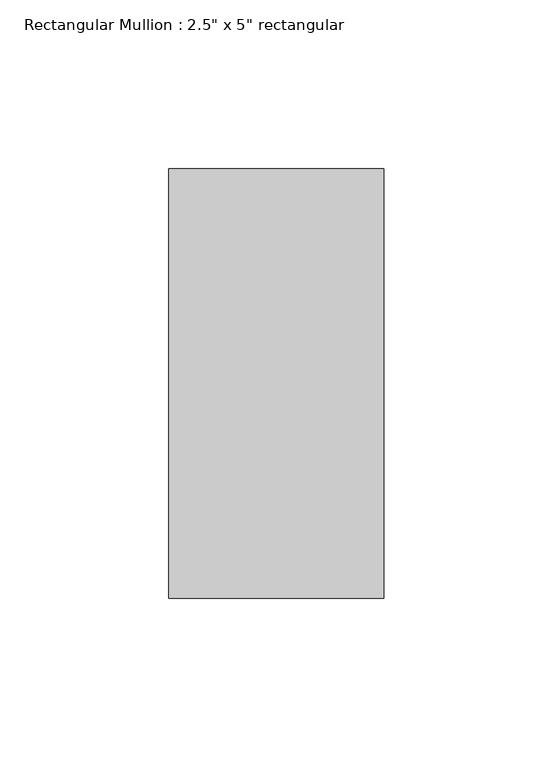
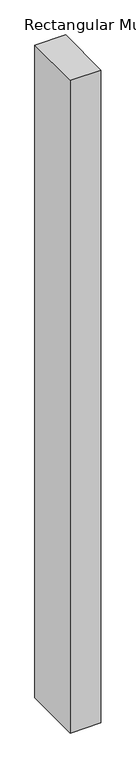
"""IFC4 building model written with IfcOpenShell, lengths in millimetres: member geometry."""

from ifc_helpers import new_model, si_unit, frame, origin, place, context, project, spatial, polyline, outline, extrude, source, transform, mapped, element, save


def member_b85431e0(model_context):
    return source(origin(), model_context, "Body", "SweptSolid", [
        extrude(outline(polyline([(31.75, 63.5), (31.75, -63.5), (-31.75, -63.5), (-31.75, 63.5), (31.75, 63.5)])), frame((0.0, 0.0, -1432.2179754), z_axis=(0.0, 0.0, 1.0), x_axis=(1.0, 0.0, 0.0)), (0.0, 0.0, 1.0), 1432.2179754),
    ])


if __name__ == "__main__":
    model = new_model("IFC4")
    model_context = context("Model", 3, world=origin())
    ifc_project = project(units=[si_unit("LENGTHUNIT", "METRE", prefix="MILLI")], contexts=[model_context])
    site = spatial("IfcSite", under=ifc_project)
    building = spatial("IfcBuilding", under=site)
    placement = place(None, origin())
    member_shape = member_b85431e0(model_context)
    element("IfcMember", 1, ObjectType="Rectangular Mullion : 2.5\" x 5\" rectangular", at=placement, inside=building, context=model_context, shape_type="MappedRepresentation", body=[
        mapped(member_shape, transform((0.0, 0.0, 0.0), x_axis=(1.0, 0.0, 0.0), y_axis=(0.0, 1.0, 0.0), z_axis=(0.0, 0.0, 1.0))),
    ])
    save(model, "model.ifc")

# Revit data of these elements
# Type "Rectangular Mullion : 2.5\" x 5\" rectangular"
#   built-in parameter 1007304 = 0.416667 (stored number, unit not read)
#   built-in parameter 1007301 = 0.104167 (stored number, unit not read)
#   built-in parameter 1007300 = 0.104167 (stored number, unit not read)
# Element 1 (IfcMember, "Rectangular Mullion : 2.5\" x 5\" rectangular")
#   Materials on its faces: "Aluminum"
# Materials
#   "Aluminum": class "Metal", colour RGB 247 247 247, transparency 0, Description = "Aluminum 6061", Cost = 0
